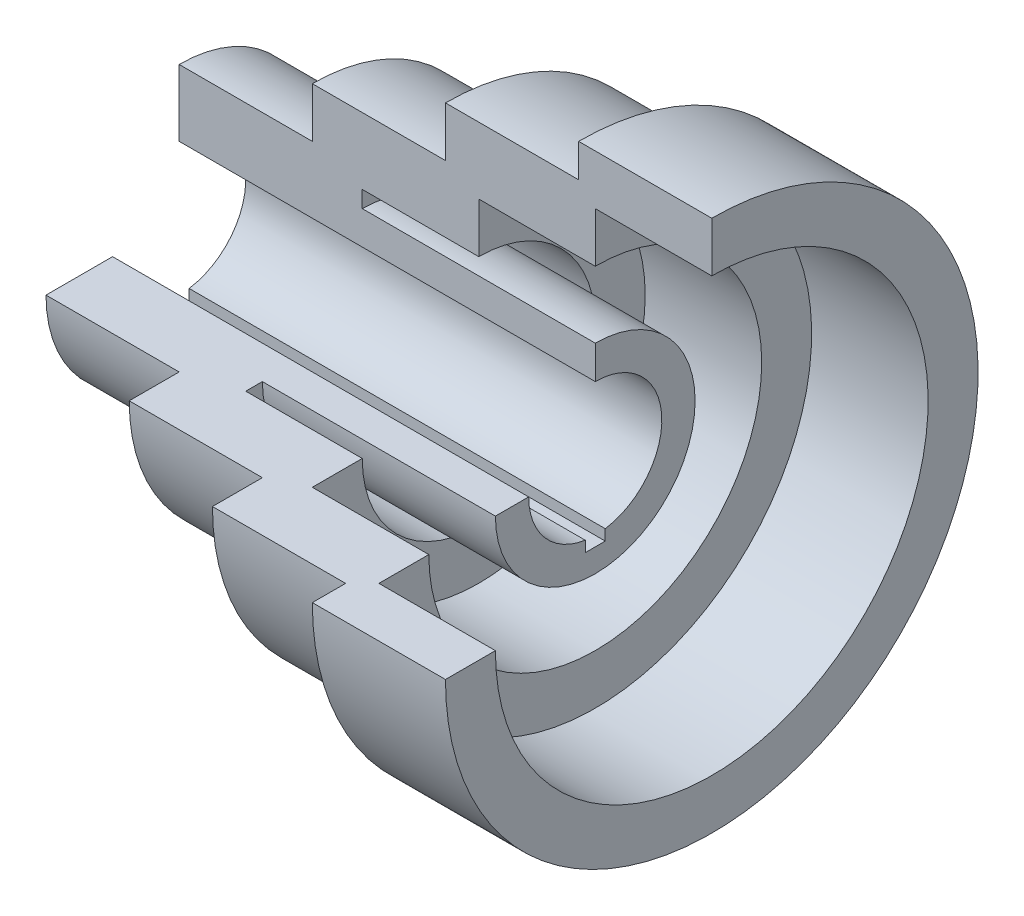
ISO-10303-21;
HEADER;
FILE_DESCRIPTION(('STEP AP214'),'2;1');
FILE_NAME('part.step','',(''),(''),'','','');
FILE_SCHEMA(('AUTOMOTIVE_DESIGN { 1 0 10303 214 1 1 1 1 }'));
ENDSEC;
DATA;
#1=APPLICATION_CONTEXT('core data for automotive mechanical design processes');
#2=APPLICATION_PROTOCOL_DEFINITION('international standard','automotive_design',2000,#1);
#3=PRODUCT_CONTEXT('',#1,'mechanical');
#4=PRODUCT('Part','Part','',(#3));
#5=PRODUCT_RELATED_PRODUCT_CATEGORY('part','',(#4));
#6=PRODUCT_DEFINITION_FORMATION('','',#4);
#7=PRODUCT_DEFINITION_CONTEXT('part definition',#1,'design');
#8=PRODUCT_DEFINITION('design','',#6,#7);
#9=PRODUCT_DEFINITION_SHAPE('','',#8);
#10=(LENGTH_UNIT() NAMED_UNIT(*) SI_UNIT(.MILLI.,.METRE.));
#11=(NAMED_UNIT(*) PLANE_ANGLE_UNIT() SI_UNIT($,.RADIAN.));
#12=(NAMED_UNIT(*) SI_UNIT($,.STERADIAN.) SOLID_ANGLE_UNIT());
#13=UNCERTAINTY_MEASURE_WITH_UNIT(LENGTH_MEASURE(1.E-05),#10,'distance_accuracy_value','');
#14=(GEOMETRIC_REPRESENTATION_CONTEXT(3) GLOBAL_UNCERTAINTY_ASSIGNED_CONTEXT((#13)) GLOBAL_UNIT_ASSIGNED_CONTEXT((#10,
#11,#12)) REPRESENTATION_CONTEXT('',''));
#15=CARTESIAN_POINT('',(0.,0.,0.));
#16=DIRECTION('',(0.,0.,1.));
#17=DIRECTION('',(1.,0.,0.));
#18=AXIS2_PLACEMENT_3D('',#15,#16,#17);
#19=CARTESIAN_POINT('',(125.,0.,0.));
#20=DIRECTION('',(1.,0.,0.));
#21=DIRECTION('',(0.,1.,0.));
#22=AXIS2_PLACEMENT_3D('',#19,#20,#21);
#23=CYLINDRICAL_SURFACE('',#22,20.);
#24=DIRECTION('',(-1.,0.,0.));
#25=VECTOR('',#24,1.);
#26=CARTESIAN_POINT('',(160.,-19.7737199332852,-3.));
#27=LINE('',#26,#25);
#28=CARTESIAN_POINT('',(125.,-19.7737199332852,-3.));
#29=VERTEX_POINT('',#28);
#30=CARTESIAN_POINT('',(0.,-19.7737199332852,-3.));
#31=VERTEX_POINT('',#30);
#32=EDGE_CURVE('E195',#29,#31,#27,.T.);
#33=ORIENTED_EDGE('',*,*,#32,.F.);
#34=CARTESIAN_POINT('',(125.,0.,0.));
#35=DIRECTION('',(1.,0.,0.));
#36=DIRECTION('',(0.,1.,0.));
#37=AXIS2_PLACEMENT_3D('',#34,#35,#36);
#38=CIRCLE('',#37,20.);
#39=CARTESIAN_POINT('',(125.,20.,0.));
#40=VERTEX_POINT('',#39);
#41=EDGE_CURVE('E219',#29,#40,#38,.T.);
#42=ORIENTED_EDGE('',*,*,#41,.T.);
#43=DIRECTION('',(1.,0.,0.));
#44=VECTOR('',#43,1.);
#45=CARTESIAN_POINT('',(0.,20.,0.));
#46=LINE('',#45,#44);
#47=CARTESIAN_POINT('',(0.,20.,0.));
#48=VERTEX_POINT('',#47);
#49=EDGE_CURVE('E212',#48,#40,#46,.T.);
#50=ORIENTED_EDGE('',*,*,#49,.F.);
#51=CARTESIAN_POINT('',(0.,0.,0.));
#52=DIRECTION('',(1.,0.,0.));
#53=DIRECTION('',(0.,1.,0.));
#54=AXIS2_PLACEMENT_3D('',#51,#52,#53);
#55=CIRCLE('',#54,20.);
#56=EDGE_CURVE('E44',#31,#48,#55,.T.);
#57=ORIENTED_EDGE('',*,*,#56,.F.);
#58=EDGE_LOOP('',(#33,#42,#50,#57));
#59=FACE_BOUND('',#58,.T.);
#60=ADVANCED_FACE('F41',(#59),#23,.F.);
#61=CARTESIAN_POINT('',(125.,0.,0.));
#62=DIRECTION('',(1.,0.,0.));
#63=DIRECTION('',(0.,1.,0.));
#64=AXIS2_PLACEMENT_3D('',#61,#62,#63);
#65=PLANE('',#64);
#66=CARTESIAN_POINT('',(125.,0.,0.));
#67=DIRECTION('',(1.,0.,0.));
#68=DIRECTION('',(0.,1.,0.));
#69=AXIS2_PLACEMENT_3D('',#66,#67,#68);
#70=CIRCLE('',#69,65.);
#71=CARTESIAN_POINT('',(125.,6.79104137598434E-13,65.));
#72=VERTEX_POINT('',#71);
#73=CARTESIAN_POINT('',(125.,65.,0.));
#74=VERTEX_POINT('',#73);
#75=EDGE_CURVE('E234',#72,#74,#70,.T.);
#76=ORIENTED_EDGE('',*,*,#75,.T.);
#77=DIRECTION('',(0.,1.,0.));
#78=VECTOR('',#77,1.);
#79=CARTESIAN_POINT('',(125.,0.,0.));
#80=LINE('',#79,#78);
#81=CARTESIAN_POINT('',(125.,50.,0.));
#82=VERTEX_POINT('',#81);
#83=EDGE_CURVE('E209',#82,#74,#80,.T.);
#84=ORIENTED_EDGE('',*,*,#83,.F.);
#85=CARTESIAN_POINT('',(125.,0.,0.));
#86=DIRECTION('',(1.,0.,0.));
#87=DIRECTION('',(0.,1.,0.));
#88=AXIS2_PLACEMENT_3D('',#85,#86,#87);
#89=CIRCLE('',#88,50.);
#90=CARTESIAN_POINT('',(125.,5.21987477350493E-13,50.));
#91=VERTEX_POINT('',#90);
#92=EDGE_CURVE('E70',#91,#82,#89,.T.);
#93=ORIENTED_EDGE('',*,*,#92,.F.);
#94=DIRECTION('',(0.,0.,1.));
#95=VECTOR('',#94,1.);
#96=CARTESIAN_POINT('',(125.,0.,0.));
#97=LINE('',#96,#95);
#98=EDGE_CURVE('E294',#91,#72,#97,.T.);
#99=ORIENTED_EDGE('',*,*,#98,.T.);
#100=EDGE_LOOP('',(#76,#84,#93,#99));
#101=FACE_BOUND('',#100,.T.);
#102=ADVANCED_FACE('F373',(#101),#65,.T.);
#103=CARTESIAN_POINT('',(125.,0.,0.));
#104=DIRECTION('',(1.,0.,0.));
#105=DIRECTION('',(0.,1.,0.));
#106=AXIS2_PLACEMENT_3D('',#103,#104,#105);
#107=CYLINDRICAL_SURFACE('',#106,65.);
#108=CARTESIAN_POINT('',(160.,0.,0.));
#109=DIRECTION('',(1.,0.,0.));
#110=DIRECTION('',(0.,1.,0.));
#111=AXIS2_PLACEMENT_3D('',#108,#109,#110);
#112=CIRCLE('',#111,65.);
#113=CARTESIAN_POINT('',(160.,6.7861841502516E-13,65.));
#114=VERTEX_POINT('',#113);
#115=CARTESIAN_POINT('',(160.,65.,0.));
#116=VERTEX_POINT('',#115);
#117=EDGE_CURVE('E240',#114,#116,#112,.T.);
#118=ORIENTED_EDGE('',*,*,#117,.T.);
#119=DIRECTION('',(1.,0.,0.));
#120=VECTOR('',#119,1.);
#121=CARTESIAN_POINT('',(0.,64.9999999999999,0.));
#122=LINE('',#121,#120);
#123=EDGE_CURVE('E403',#74,#116,#122,.T.);
#124=ORIENTED_EDGE('',*,*,#123,.F.);
#125=ORIENTED_EDGE('',*,*,#75,.F.);
#126=DIRECTION('',(1.,0.,0.));
#127=VECTOR('',#126,1.);
#128=CARTESIAN_POINT('',(0.,6.8083886107441E-13,64.9999999999999));
#129=LINE('',#128,#127);
#130=EDGE_CURVE('E299',#72,#114,#129,.T.);
#131=ORIENTED_EDGE('',*,*,#130,.T.);
#132=EDGE_LOOP('',(#118,#124,#125,#131));
#133=FACE_BOUND('',#132,.T.);
#134=ADVANCED_FACE('F43',(#133),#107,.F.);
#135=CARTESIAN_POINT('',(160.,0.,0.));
#136=DIRECTION('',(-1.,0.,0.));
#137=DIRECTION('',(0.,-1.,0.));
#138=AXIS2_PLACEMENT_3D('',#135,#136,#137);
#139=PLANE('',#138);
#140=CARTESIAN_POINT('',(160.,0.,0.));
#141=DIRECTION('',(1.,0.,0.));
#142=DIRECTION('',(0.,1.,0.));
#143=AXIS2_PLACEMENT_3D('',#140,#141,#142);
#144=CIRCLE('',#143,80.);
#145=CARTESIAN_POINT('',(160.,8.35735075273101E-13,80.));
#146=VERTEX_POINT('',#145);
#147=CARTESIAN_POINT('',(160.,80.,0.));
#148=VERTEX_POINT('',#147);
#149=EDGE_CURVE('E239',#146,#148,#144,.T.);
#150=ORIENTED_EDGE('',*,*,#149,.T.);
#151=DIRECTION('',(0.,-1.,0.));
#152=VECTOR('',#151,1.);
#153=CARTESIAN_POINT('',(160.,0.,0.));
#154=LINE('',#153,#152);
#155=EDGE_CURVE('E406',#148,#116,#154,.T.);
#156=ORIENTED_EDGE('',*,*,#155,.T.);
#157=ORIENTED_EDGE('',*,*,#117,.F.);
#158=DIRECTION('',(0.,0.,-1.));
#159=VECTOR('',#158,1.);
#160=CARTESIAN_POINT('',(160.,0.,0.));
#161=LINE('',#160,#159);
#162=EDGE_CURVE('E298',#146,#114,#161,.T.);
#163=ORIENTED_EDGE('',*,*,#162,.F.);
#164=EDGE_LOOP('',(#150,#156,#157,#163));
#165=FACE_BOUND('',#164,.T.);
#166=ADVANCED_FACE('F455',(#165),#139,.F.);
#167=CARTESIAN_POINT('',(125.,0.,0.));
#168=DIRECTION('',(1.,0.,0.));
#169=DIRECTION('',(0.,1.,0.));
#170=AXIS2_PLACEMENT_3D('',#167,#168,#169);
#171=CYLINDRICAL_SURFACE('',#170,80.);
#172=CARTESIAN_POINT('',(120.,0.,0.));
#173=DIRECTION('',(1.,0.,0.));
#174=DIRECTION('',(0.,1.,0.));
#175=AXIS2_PLACEMENT_3D('',#172,#173,#174);
#176=CIRCLE('',#175,80.);
#177=CARTESIAN_POINT('',(120.,8.36290186785414E-13,80.));
#178=VERTEX_POINT('',#177);
#179=CARTESIAN_POINT('',(120.,80.,0.));
#180=VERTEX_POINT('',#179);
#181=EDGE_CURVE('E244',#178,#180,#176,.T.);
#182=ORIENTED_EDGE('',*,*,#181,.T.);
#183=DIRECTION('',(1.,0.,0.));
#184=VECTOR('',#183,1.);
#185=CARTESIAN_POINT('',(0.,79.9999999999999,0.));
#186=LINE('',#185,#184);
#187=EDGE_CURVE('E412',#180,#148,#186,.T.);
#188=ORIENTED_EDGE('',*,*,#187,.T.);
#189=ORIENTED_EDGE('',*,*,#149,.F.);
#190=DIRECTION('',(1.,0.,0.));
#191=VECTOR('',#190,1.);
#192=CARTESIAN_POINT('',(0.,8.37955521322351E-13,79.9999999999999));
#193=LINE('',#192,#191);
#194=EDGE_CURVE('E305',#178,#146,#193,.T.);
#195=ORIENTED_EDGE('',*,*,#194,.F.);
#196=EDGE_LOOP('',(#182,#188,#189,#195));
#197=FACE_BOUND('',#196,.T.);
#198=ADVANCED_FACE('F450',(#197),#171,.T.);
#199=CARTESIAN_POINT('',(120.,0.,0.));
#200=DIRECTION('',(1.,0.,0.));
#201=DIRECTION('',(0.,1.,0.));
#202=AXIS2_PLACEMENT_3D('',#199,#200,#201);
#203=PLANE('',#202);
#204=CARTESIAN_POINT('',(120.,0.,0.));
#205=DIRECTION('',(1.,0.,0.));
#206=DIRECTION('',(0.,1.,0.));
#207=AXIS2_PLACEMENT_3D('',#204,#205,#206);
#208=CIRCLE('',#207,70.);
#209=CARTESIAN_POINT('',(120.,7.3154574662012E-13,70.));
#210=VERTEX_POINT('',#209);
#211=CARTESIAN_POINT('',(120.,70.,0.));
#212=VERTEX_POINT('',#211);
#213=EDGE_CURVE('E245',#210,#212,#208,.T.);
#214=ORIENTED_EDGE('',*,*,#213,.T.);
#215=DIRECTION('',(0.,1.,0.));
#216=VECTOR('',#215,1.);
#217=CARTESIAN_POINT('',(120.,0.,0.));
#218=LINE('',#217,#216);
#219=EDGE_CURVE('E417',#212,#180,#218,.T.);
#220=ORIENTED_EDGE('',*,*,#219,.T.);
#221=ORIENTED_EDGE('',*,*,#181,.F.);
#222=DIRECTION('',(0.,0.,1.));
#223=VECTOR('',#222,1.);
#224=CARTESIAN_POINT('',(120.,0.,0.));
#225=LINE('',#224,#223);
#226=EDGE_CURVE('E304',#210,#178,#225,.T.);
#227=ORIENTED_EDGE('',*,*,#226,.F.);
#228=EDGE_LOOP('',(#214,#220,#221,#227));
#229=FACE_BOUND('',#228,.T.);
#230=ADVANCED_FACE('F444',(#229),#203,.F.);
#231=CARTESIAN_POINT('',(125.,0.,0.));
#232=DIRECTION('',(1.,0.,0.));
#233=DIRECTION('',(0.,1.,0.));
#234=AXIS2_PLACEMENT_3D('',#231,#232,#233);
#235=CYLINDRICAL_SURFACE('',#234,70.);
#236=CARTESIAN_POINT('',(80.,0.,0.));
#237=DIRECTION('',(1.,0.,0.));
#238=DIRECTION('',(0.,1.,0.));
#239=AXIS2_PLACEMENT_3D('',#236,#237,#238);
#240=CIRCLE('',#239,70.);
#241=CARTESIAN_POINT('',(80.,7.32100858132433E-13,70.));
#242=VERTEX_POINT('',#241);
#243=CARTESIAN_POINT('',(80.,70.,0.));
#244=VERTEX_POINT('',#243);
#245=EDGE_CURVE('E242',#242,#244,#240,.T.);
#246=ORIENTED_EDGE('',*,*,#245,.T.);
#247=DIRECTION('',(1.,0.,0.));
#248=VECTOR('',#247,1.);
#249=CARTESIAN_POINT('',(0.,69.9999999999999,0.));
#250=LINE('',#249,#248);
#251=EDGE_CURVE('E419',#244,#212,#250,.T.);
#252=ORIENTED_EDGE('',*,*,#251,.T.);
#253=ORIENTED_EDGE('',*,*,#213,.F.);
#254=DIRECTION('',(1.,0.,0.));
#255=VECTOR('',#254,1.);
#256=CARTESIAN_POINT('',(0.,7.33211081157057E-13,69.9999999999999));
#257=LINE('',#256,#255);
#258=EDGE_CURVE('E306',#242,#210,#257,.T.);
#259=ORIENTED_EDGE('',*,*,#258,.F.);
#260=EDGE_LOOP('',(#246,#252,#253,#259));
#261=FACE_BOUND('',#260,.T.);
#262=ADVANCED_FACE('F438',(#261),#235,.T.);
#263=CARTESIAN_POINT('',(80.,0.,0.));
#264=DIRECTION('',(1.,0.,0.));
#265=DIRECTION('',(0.,1.,0.));
#266=AXIS2_PLACEMENT_3D('',#263,#264,#265);
#267=PLANE('',#266);
#268=CARTESIAN_POINT('',(80.,0.,0.));
#269=DIRECTION('',(1.,0.,0.));
#270=DIRECTION('',(0.,1.,0.));
#271=AXIS2_PLACEMENT_3D('',#268,#269,#270);
#272=CIRCLE('',#271,55.);
#273=CARTESIAN_POINT('',(80.,5.74984197884491E-13,55.));
#274=VERTEX_POINT('',#273);
#275=CARTESIAN_POINT('',(80.,55.,0.));
#276=VERTEX_POINT('',#275);
#277=EDGE_CURVE('E250',#274,#276,#272,.T.);
#278=ORIENTED_EDGE('',*,*,#277,.T.);
#279=DIRECTION('',(0.,1.,0.));
#280=VECTOR('',#279,1.);
#281=CARTESIAN_POINT('',(80.,0.,0.));
#282=LINE('',#281,#280);
#283=EDGE_CURVE('E421',#276,#244,#282,.T.);
#284=ORIENTED_EDGE('',*,*,#283,.T.);
#285=ORIENTED_EDGE('',*,*,#245,.F.);
#286=DIRECTION('',(0.,0.,1.));
#287=VECTOR('',#286,1.);
#288=CARTESIAN_POINT('',(80.,0.,0.));
#289=LINE('',#288,#287);
#290=EDGE_CURVE('E313',#274,#242,#289,.T.);
#291=ORIENTED_EDGE('',*,*,#290,.F.);
#292=EDGE_LOOP('',(#278,#284,#285,#291));
#293=FACE_BOUND('',#292,.T.);
#294=ADVANCED_FACE('F434',(#293),#267,.F.);
#295=CARTESIAN_POINT('',(125.,0.,0.));
#296=DIRECTION('',(1.,0.,0.));
#297=DIRECTION('',(0.,1.,0.));
#298=AXIS2_PLACEMENT_3D('',#295,#296,#297);
#299=CYLINDRICAL_SURFACE('',#298,55.);
#300=CARTESIAN_POINT('',(40.,0.,0.));
#301=DIRECTION('',(1.,0.,0.));
#302=DIRECTION('',(0.,1.,0.));
#303=AXIS2_PLACEMENT_3D('',#300,#301,#302);
#304=CIRCLE('',#303,55.);
#305=CARTESIAN_POINT('',(40.,5.75539309396804E-13,55.));
#306=VERTEX_POINT('',#305);
#307=CARTESIAN_POINT('',(40.,55.,0.));
#308=VERTEX_POINT('',#307);
#309=EDGE_CURVE('E247',#306,#308,#304,.T.);
#310=ORIENTED_EDGE('',*,*,#309,.T.);
#311=DIRECTION('',(1.,0.,0.));
#312=VECTOR('',#311,1.);
#313=CARTESIAN_POINT('',(0.,55.,0.));
#314=LINE('',#313,#312);
#315=EDGE_CURVE('E426',#308,#276,#314,.T.);
#316=ORIENTED_EDGE('',*,*,#315,.T.);
#317=ORIENTED_EDGE('',*,*,#277,.F.);
#318=DIRECTION('',(1.,0.,0.));
#319=VECTOR('',#318,1.);
#320=CARTESIAN_POINT('',(0.,5.76094420909117E-13,55.));
#321=LINE('',#320,#319);
#322=EDGE_CURVE('E314',#306,#274,#321,.T.);
#323=ORIENTED_EDGE('',*,*,#322,.F.);
#324=EDGE_LOOP('',(#310,#316,#317,#323));
#325=FACE_BOUND('',#324,.T.);
#326=ADVANCED_FACE('F431',(#325),#299,.T.);
#327=CARTESIAN_POINT('',(40.,0.,0.));
#328=DIRECTION('',(1.,0.,0.));
#329=DIRECTION('',(0.,1.,0.));
#330=AXIS2_PLACEMENT_3D('',#327,#328,#329);
#331=PLANE('',#330);
#332=CARTESIAN_POINT('',(40.,0.,0.));
#333=DIRECTION('',(1.,0.,0.));
#334=DIRECTION('',(0.,1.,0.));
#335=AXIS2_PLACEMENT_3D('',#332,#333,#334);
#336=CIRCLE('',#335,40.);
#337=CARTESIAN_POINT('',(40.,4.18422649148863E-13,40.));
#338=VERTEX_POINT('',#337);
#339=CARTESIAN_POINT('',(40.,40.,0.));
#340=VERTEX_POINT('',#339);
#341=EDGE_CURVE('E249',#338,#340,#336,.T.);
#342=ORIENTED_EDGE('',*,*,#341,.T.);
#343=DIRECTION('',(0.,1.,0.));
#344=VECTOR('',#343,1.);
#345=CARTESIAN_POINT('',(40.,0.,0.));
#346=LINE('',#345,#344);
#347=EDGE_CURVE('E269',#340,#308,#346,.T.);
#348=ORIENTED_EDGE('',*,*,#347,.T.);
#349=ORIENTED_EDGE('',*,*,#309,.F.);
#350=DIRECTION('',(0.,0.,1.));
#351=VECTOR('',#350,1.);
#352=CARTESIAN_POINT('',(40.,0.,0.));
#353=LINE('',#352,#351);
#354=EDGE_CURVE('E320',#338,#306,#353,.T.);
#355=ORIENTED_EDGE('',*,*,#354,.F.);
#356=EDGE_LOOP('',(#342,#348,#349,#355));
#357=FACE_BOUND('',#356,.T.);
#358=ADVANCED_FACE('F428',(#357),#331,.F.);
#359=CARTESIAN_POINT('',(125.,0.,0.));
#360=DIRECTION('',(1.,0.,0.));
#361=DIRECTION('',(0.,1.,0.));
#362=AXIS2_PLACEMENT_3D('',#359,#360,#361);
#363=CYLINDRICAL_SURFACE('',#362,40.);
#364=CARTESIAN_POINT('',(0.,0.,0.));
#365=DIRECTION('',(1.,0.,0.));
#366=DIRECTION('',(0.,1.,0.));
#367=AXIS2_PLACEMENT_3D('',#364,#365,#366);
#368=CIRCLE('',#367,40.);
#369=CARTESIAN_POINT('',(0.,4.18977760661176E-13,40.));
#370=VERTEX_POINT('',#369);
#371=CARTESIAN_POINT('',(0.,40.,0.));
#372=VERTEX_POINT('',#371);
#373=EDGE_CURVE('E217',#370,#372,#368,.T.);
#374=ORIENTED_EDGE('',*,*,#373,.T.);
#375=DIRECTION('',(1.,0.,0.));
#376=VECTOR('',#375,1.);
#377=CARTESIAN_POINT('',(0.,40.,0.));
#378=LINE('',#377,#376);
#379=EDGE_CURVE('E257',#372,#340,#378,.T.);
#380=ORIENTED_EDGE('',*,*,#379,.T.);
#381=ORIENTED_EDGE('',*,*,#341,.F.);
#382=DIRECTION('',(1.,0.,0.));
#383=VECTOR('',#382,1.);
#384=CARTESIAN_POINT('',(0.,4.18977760661176E-13,40.));
#385=LINE('',#384,#383);
#386=EDGE_CURVE('E265',#370,#338,#385,.T.);
#387=ORIENTED_EDGE('',*,*,#386,.F.);
#388=EDGE_LOOP('',(#374,#380,#381,#387));
#389=FACE_BOUND('',#388,.T.);
#390=ADVANCED_FACE('F259',(#389),#363,.T.);
#391=CARTESIAN_POINT('',(0.,0.,0.));
#392=DIRECTION('',(1.,0.,0.));
#393=DIRECTION('',(0.,1.,0.));
#394=AXIS2_PLACEMENT_3D('',#391,#392,#393);
#395=PLANE('',#394);
#396=DIRECTION('',(0.,0.,-1.));
#397=VECTOR('',#396,1.);
#398=CARTESIAN_POINT('',(0.,-23.,0.));
#399=LINE('',#398,#397);
#400=CARTESIAN_POINT('',(0.,-23.,3.));
#401=VERTEX_POINT('',#400);
#402=CARTESIAN_POINT('',(0.,-23.,-3.));
#403=VERTEX_POINT('',#402);
#404=EDGE_CURVE('E207',#401,#403,#399,.T.);
#405=ORIENTED_EDGE('',*,*,#404,.T.);
#406=DIRECTION('',(0.,1.,0.));
#407=VECTOR('',#406,1.);
#408=CARTESIAN_POINT('',(0.,0.,-3.));
#409=LINE('',#408,#407);
#410=EDGE_CURVE('E198',#403,#31,#409,.T.);
#411=ORIENTED_EDGE('',*,*,#410,.T.);
#412=ORIENTED_EDGE('',*,*,#56,.T.);
#413=DIRECTION('',(0.,1.,0.));
#414=VECTOR('',#413,1.);
#415=CARTESIAN_POINT('',(0.,0.,0.));
#416=LINE('',#415,#414);
#417=EDGE_CURVE('E268',#48,#372,#416,.T.);
#418=ORIENTED_EDGE('',*,*,#417,.T.);
#419=ORIENTED_EDGE('',*,*,#373,.F.);
#420=DIRECTION('',(0.,0.,1.));
#421=VECTOR('',#420,1.);
#422=CARTESIAN_POINT('',(0.,0.,0.));
#423=LINE('',#422,#421);
#424=CARTESIAN_POINT('',(0.,2.09488880330588E-13,20.));
#425=VERTEX_POINT('',#424);
#426=EDGE_CURVE('E321',#425,#370,#423,.T.);
#427=ORIENTED_EDGE('',*,*,#426,.F.);
#428=CARTESIAN_POINT('',(-6.E-06,-19.7737199332852,3.));
#429=VERTEX_POINT('',#428);
#430=EDGE_CURVE('E214',#425,#429,#55,.T.);
#431=ORIENTED_EDGE('',*,*,#430,.T.);
#432=DIRECTION('',(0.,-1.,0.));
#433=VECTOR('',#432,1.);
#434=CARTESIAN_POINT('',(0.,0.,3.));
#435=LINE('',#434,#433);
#436=EDGE_CURVE('E390',#429,#401,#435,.T.);
#437=ORIENTED_EDGE('',*,*,#436,.T.);
#438=EDGE_LOOP('',(#405,#411,#412,#418,#419,#427,#431,#437));
#439=FACE_BOUND('',#438,.T.);
#440=ADVANCED_FACE('F202',(#439),#395,.F.);
#441=DIRECTION('',(-1.,0.,0.));
#442=VECTOR('',#441,1.);
#443=CARTESIAN_POINT('',(160.,-19.7737199332852,3.));
#444=LINE('',#443,#442);
#445=CARTESIAN_POINT('',(125.,-19.7737199332852,3.));
#446=VERTEX_POINT('',#445);
#447=EDGE_CURVE('E56',#446,#429,#444,.T.);
#448=ORIENTED_EDGE('',*,*,#447,.T.);
#449=ORIENTED_EDGE('',*,*,#430,.F.);
#450=DIRECTION('',(1.,0.,0.));
#451=VECTOR('',#450,1.);
#452=CARTESIAN_POINT('',(0.,2.09488880330588E-13,20.));
#453=LINE('',#452,#451);
#454=CARTESIAN_POINT('',(125.,2.07754156854611E-13,20.));
#455=VERTEX_POINT('',#454);
#456=EDGE_CURVE('E323',#425,#455,#453,.T.);
#457=ORIENTED_EDGE('',*,*,#456,.T.);
#458=EDGE_CURVE('E216',#455,#446,#38,.T.);
#459=ORIENTED_EDGE('',*,*,#458,.T.);
#460=EDGE_LOOP('',(#448,#449,#457,#459));
#461=FACE_BOUND('',#460,.T.);
#462=ADVANCED_FACE('F367',(#461),#23,.F.);
#463=CARTESIAN_POINT('',(125.,0.,0.));
#464=DIRECTION('',(1.,0.,0.));
#465=DIRECTION('',(0.,1.,0.));
#466=AXIS2_PLACEMENT_3D('',#463,#464,#465);
#467=PLANE('',#466);
#468=DIRECTION('',(0.,1.,0.));
#469=VECTOR('',#468,1.);
#470=CARTESIAN_POINT('',(125.,0.,-3.));
#471=LINE('',#470,#469);
#472=CARTESIAN_POINT('',(125.,-23.,-3.));
#473=VERTEX_POINT('',#472);
#474=EDGE_CURVE('E11',#473,#29,#471,.T.);
#475=ORIENTED_EDGE('',*,*,#474,.F.);
#476=DIRECTION('',(0.,0.,-1.));
#477=VECTOR('',#476,1.);
#478=CARTESIAN_POINT('',(125.,-23.,0.));
#479=LINE('',#478,#477);
#480=CARTESIAN_POINT('',(125.,-23.,3.));
#481=VERTEX_POINT('',#480);
#482=EDGE_CURVE('E51',#481,#473,#479,.T.);
#483=ORIENTED_EDGE('',*,*,#482,.F.);
#484=DIRECTION('',(0.,-1.,0.));
#485=VECTOR('',#484,1.);
#486=CARTESIAN_POINT('',(125.,0.,3.));
#487=LINE('',#486,#485);
#488=EDGE_CURVE('E233',#446,#481,#487,.T.);
#489=ORIENTED_EDGE('',*,*,#488,.F.);
#490=ORIENTED_EDGE('',*,*,#458,.F.);
#491=DIRECTION('',(0.,0.,1.));
#492=VECTOR('',#491,1.);
#493=CARTESIAN_POINT('',(125.,0.,0.));
#494=LINE('',#493,#492);
#495=CARTESIAN_POINT('',(125.,3.12498597019905E-13,30.));
#496=VERTEX_POINT('',#495);
#497=EDGE_CURVE('E324',#455,#496,#494,.T.);
#498=ORIENTED_EDGE('',*,*,#497,.T.);
#499=CARTESIAN_POINT('',(125.,0.,0.));
#500=DIRECTION('',(1.,0.,0.));
#501=DIRECTION('',(0.,1.,0.));
#502=AXIS2_PLACEMENT_3D('',#499,#500,#501);
#503=CIRCLE('',#502,30.);
#504=CARTESIAN_POINT('',(125.,30.,0.));
#505=VERTEX_POINT('',#504);
#506=EDGE_CURVE('E221',#496,#505,#503,.T.);
#507=ORIENTED_EDGE('',*,*,#506,.T.);
#508=DIRECTION('',(0.,1.,0.));
#509=VECTOR('',#508,1.);
#510=CARTESIAN_POINT('',(125.,0.,0.));
#511=LINE('',#510,#509);
#512=EDGE_CURVE('E272',#40,#505,#511,.T.);
#513=ORIENTED_EDGE('',*,*,#512,.F.);
#514=ORIENTED_EDGE('',*,*,#41,.F.);
#515=EDGE_LOOP('',(#475,#483,#489,#490,#498,#507,#513,#514));
#516=FACE_BOUND('',#515,.T.);
#517=ADVANCED_FACE('F353',(#516),#467,.T.);
#518=CARTESIAN_POINT('',(125.,0.,0.));
#519=DIRECTION('',(1.,0.,0.));
#520=DIRECTION('',(0.,1.,0.));
#521=AXIS2_PLACEMENT_3D('',#518,#519,#520);
#522=CYLINDRICAL_SURFACE('',#521,30.);
#523=CARTESIAN_POINT('',(55.,0.,0.));
#524=DIRECTION('',(1.,0.,0.));
#525=DIRECTION('',(0.,1.,0.));
#526=AXIS2_PLACEMENT_3D('',#523,#524,#525);
#527=CIRCLE('',#526,30.);
#528=CARTESIAN_POINT('',(55.,3.13470042166452E-13,30.));
#529=VERTEX_POINT('',#528);
#530=CARTESIAN_POINT('',(55.,30.,0.));
#531=VERTEX_POINT('',#530);
#532=EDGE_CURVE('E349',#529,#531,#527,.T.);
#533=ORIENTED_EDGE('',*,*,#532,.T.);
#534=DIRECTION('',(-1.,0.,0.));
#535=VECTOR('',#534,1.);
#536=CARTESIAN_POINT('',(0.,30.,0.));
#537=LINE('',#536,#535);
#538=EDGE_CURVE('E276',#505,#531,#537,.T.);
#539=ORIENTED_EDGE('',*,*,#538,.F.);
#540=ORIENTED_EDGE('',*,*,#506,.F.);
#541=DIRECTION('',(-1.,0.,0.));
#542=VECTOR('',#541,1.);
#543=CARTESIAN_POINT('',(0.,3.14233320495881E-13,30.));
#544=LINE('',#543,#542);
#545=EDGE_CURVE('E327',#496,#529,#544,.T.);
#546=ORIENTED_EDGE('',*,*,#545,.T.);
#547=EDGE_LOOP('',(#533,#539,#540,#546));
#548=FACE_BOUND('',#547,.T.);
#549=ADVANCED_FACE('F358',(#548),#522,.T.);
#550=CARTESIAN_POINT('',(55.,0.,0.));
#551=DIRECTION('',(1.,0.,0.));
#552=DIRECTION('',(0.,1.,0.));
#553=AXIS2_PLACEMENT_3D('',#550,#551,#552);
#554=PLANE('',#553);
#555=CARTESIAN_POINT('',(55.,0.,0.));
#556=DIRECTION('',(1.,0.,0.));
#557=DIRECTION('',(0.,1.,0.));
#558=AXIS2_PLACEMENT_3D('',#555,#556,#557);
#559=CIRCLE('',#558,35.);
#560=CARTESIAN_POINT('',(55.,3.65842262249099E-13,35.));
#561=VERTEX_POINT('',#560);
#562=CARTESIAN_POINT('',(55.,35.,0.));
#563=VERTEX_POINT('',#562);
#564=EDGE_CURVE('E346',#561,#563,#559,.T.);
#565=ORIENTED_EDGE('',*,*,#564,.T.);
#566=DIRECTION('',(0.,1.,0.));
#567=VECTOR('',#566,1.);
#568=CARTESIAN_POINT('',(55.,0.,0.));
#569=LINE('',#568,#567);
#570=EDGE_CURVE('E281',#531,#563,#569,.T.);
#571=ORIENTED_EDGE('',*,*,#570,.F.);
#572=ORIENTED_EDGE('',*,*,#532,.F.);
#573=DIRECTION('',(0.,0.,1.));
#574=VECTOR('',#573,1.);
#575=CARTESIAN_POINT('',(55.,0.,0.));
#576=LINE('',#575,#574);
#577=EDGE_CURVE('E332',#529,#561,#576,.T.);
#578=ORIENTED_EDGE('',*,*,#577,.T.);
#579=EDGE_LOOP('',(#565,#571,#572,#578));
#580=FACE_BOUND('',#579,.T.);
#581=ADVANCED_FACE('F359',(#580),#554,.T.);
#582=CARTESIAN_POINT('',(125.,0.,0.));
#583=DIRECTION('',(1.,0.,0.));
#584=DIRECTION('',(0.,1.,0.));
#585=AXIS2_PLACEMENT_3D('',#582,#583,#584);
#586=CYLINDRICAL_SURFACE('',#585,35.);
#587=CARTESIAN_POINT('',(90.,0.,0.));
#588=DIRECTION('',(1.,0.,0.));
#589=DIRECTION('',(0.,1.,0.));
#590=AXIS2_PLACEMENT_3D('',#587,#588,#589);
#591=CIRCLE('',#590,35.);
#592=CARTESIAN_POINT('',(90.,3.65356539675825E-13,35.));
#593=VERTEX_POINT('',#592);
#594=CARTESIAN_POINT('',(90.,35.,0.));
#595=VERTEX_POINT('',#594);
#596=EDGE_CURVE('E347',#593,#595,#591,.T.);
#597=ORIENTED_EDGE('',*,*,#596,.T.);
#598=DIRECTION('',(1.,0.,0.));
#599=VECTOR('',#598,1.);
#600=CARTESIAN_POINT('',(0.,35.,0.));
#601=LINE('',#600,#599);
#602=EDGE_CURVE('E282',#563,#595,#601,.T.);
#603=ORIENTED_EDGE('',*,*,#602,.F.);
#604=ORIENTED_EDGE('',*,*,#564,.F.);
#605=DIRECTION('',(1.,0.,0.));
#606=VECTOR('',#605,1.);
#607=CARTESIAN_POINT('',(0.,3.66605540578529E-13,35.));
#608=LINE('',#607,#606);
#609=EDGE_CURVE('E331',#561,#593,#608,.T.);
#610=ORIENTED_EDGE('',*,*,#609,.T.);
#611=EDGE_LOOP('',(#597,#603,#604,#610));
#612=FACE_BOUND('',#611,.T.);
#613=ADVANCED_FACE('F368',(#612),#586,.F.);
#614=CARTESIAN_POINT('',(90.,0.,0.));
#615=DIRECTION('',(1.,0.,0.));
#616=DIRECTION('',(0.,1.,0.));
#617=AXIS2_PLACEMENT_3D('',#614,#615,#616);
#618=PLANE('',#617);
#619=CARTESIAN_POINT('',(90.,0.,0.));
#620=DIRECTION('',(1.,0.,0.));
#621=DIRECTION('',(0.,1.,0.));
#622=AXIS2_PLACEMENT_3D('',#619,#620,#621);
#623=CIRCLE('',#622,50.);
#624=CARTESIAN_POINT('',(90.,5.22473199923766E-13,50.));
#625=VERTEX_POINT('',#624);
#626=CARTESIAN_POINT('',(90.,50.,0.));
#627=VERTEX_POINT('',#626);
#628=EDGE_CURVE('E342',#625,#627,#623,.T.);
#629=ORIENTED_EDGE('',*,*,#628,.T.);
#630=DIRECTION('',(0.,1.,0.));
#631=VECTOR('',#630,1.);
#632=CARTESIAN_POINT('',(90.,0.,0.));
#633=LINE('',#632,#631);
#634=EDGE_CURVE('E288',#595,#627,#633,.T.);
#635=ORIENTED_EDGE('',*,*,#634,.F.);
#636=ORIENTED_EDGE('',*,*,#596,.F.);
#637=DIRECTION('',(0.,0.,1.));
#638=VECTOR('',#637,1.);
#639=CARTESIAN_POINT('',(90.,0.,0.));
#640=LINE('',#639,#638);
#641=EDGE_CURVE('E336',#593,#625,#640,.T.);
#642=ORIENTED_EDGE('',*,*,#641,.T.);
#643=EDGE_LOOP('',(#629,#635,#636,#642));
#644=FACE_BOUND('',#643,.T.);
#645=ADVANCED_FACE('F398',(#644),#618,.T.);
#646=CARTESIAN_POINT('',(125.,0.,0.));
#647=DIRECTION('',(1.,0.,0.));
#648=DIRECTION('',(0.,1.,0.));
#649=AXIS2_PLACEMENT_3D('',#646,#647,#648);
#650=CYLINDRICAL_SURFACE('',#649,50.);
#651=DIRECTION('',(1.,0.,0.));
#652=VECTOR('',#651,1.);
#653=CARTESIAN_POINT('',(0.,5.2372220082647E-13,50.));
#654=LINE('',#653,#652);
#655=EDGE_CURVE('E337',#625,#91,#654,.T.);
#656=ORIENTED_EDGE('',*,*,#655,.T.);
#657=ORIENTED_EDGE('',*,*,#92,.T.);
#658=DIRECTION('',(1.,0.,0.));
#659=VECTOR('',#658,1.);
#660=CARTESIAN_POINT('',(0.,50.,0.));
#661=LINE('',#660,#659);
#662=EDGE_CURVE('E292',#627,#82,#661,.T.);
#663=ORIENTED_EDGE('',*,*,#662,.F.);
#664=ORIENTED_EDGE('',*,*,#628,.F.);
#665=EDGE_LOOP('',(#656,#657,#663,#664));
#666=FACE_BOUND('',#665,.T.);
#667=ADVANCED_FACE('F405',(#666),#650,.F.);
#668=CARTESIAN_POINT('',(0.,0.,0.));
#669=DIRECTION('',(0.,-1.,0.));
#670=DIRECTION('',(1.,0.,0.));
#671=AXIS2_PLACEMENT_3D('',#668,#669,#670);
#672=PLANE('',#671);
#673=ORIENTED_EDGE('',*,*,#98,.F.);
#674=ORIENTED_EDGE('',*,*,#655,.F.);
#675=ORIENTED_EDGE('',*,*,#641,.F.);
#676=ORIENTED_EDGE('',*,*,#609,.F.);
#677=ORIENTED_EDGE('',*,*,#577,.F.);
#678=ORIENTED_EDGE('',*,*,#545,.F.);
#679=ORIENTED_EDGE('',*,*,#497,.F.);
#680=ORIENTED_EDGE('',*,*,#456,.F.);
#681=ORIENTED_EDGE('',*,*,#426,.T.);
#682=ORIENTED_EDGE('',*,*,#386,.T.);
#683=ORIENTED_EDGE('',*,*,#354,.T.);
#684=ORIENTED_EDGE('',*,*,#322,.T.);
#685=ORIENTED_EDGE('',*,*,#290,.T.);
#686=ORIENTED_EDGE('',*,*,#258,.T.);
#687=ORIENTED_EDGE('',*,*,#226,.T.);
#688=ORIENTED_EDGE('',*,*,#194,.T.);
#689=ORIENTED_EDGE('',*,*,#162,.T.);
#690=ORIENTED_EDGE('',*,*,#130,.F.);
#691=EDGE_LOOP('',(#673,#674,#675,#676,#677,#678,#679,#680,#681,#682,#683,#684,#685,#686,#687,
#688,#689,#690));
#692=FACE_BOUND('',#691,.T.);
#693=ADVANCED_FACE('F388',(#692),#672,.F.);
#694=CARTESIAN_POINT('',(0.,0.,0.));
#695=DIRECTION('',(0.,0.,1.));
#696=DIRECTION('',(1.,0.,0.));
#697=AXIS2_PLACEMENT_3D('',#694,#695,#696);
#698=PLANE('',#697);
#699=ORIENTED_EDGE('',*,*,#83,.T.);
#700=ORIENTED_EDGE('',*,*,#123,.T.);
#701=ORIENTED_EDGE('',*,*,#155,.F.);
#702=ORIENTED_EDGE('',*,*,#187,.F.);
#703=ORIENTED_EDGE('',*,*,#219,.F.);
#704=ORIENTED_EDGE('',*,*,#251,.F.);
#705=ORIENTED_EDGE('',*,*,#283,.F.);
#706=ORIENTED_EDGE('',*,*,#315,.F.);
#707=ORIENTED_EDGE('',*,*,#347,.F.);
#708=ORIENTED_EDGE('',*,*,#379,.F.);
#709=ORIENTED_EDGE('',*,*,#417,.F.);
#710=ORIENTED_EDGE('',*,*,#49,.T.);
#711=ORIENTED_EDGE('',*,*,#512,.T.);
#712=ORIENTED_EDGE('',*,*,#538,.T.);
#713=ORIENTED_EDGE('',*,*,#570,.T.);
#714=ORIENTED_EDGE('',*,*,#602,.T.);
#715=ORIENTED_EDGE('',*,*,#634,.T.);
#716=ORIENTED_EDGE('',*,*,#662,.T.);
#717=EDGE_LOOP('',(#699,#700,#701,#702,#703,#704,#705,#706,#707,#708,#709,#710,#711,#712,#713,
#714,#715,#716));
#718=FACE_BOUND('',#717,.T.);
#719=ADVANCED_FACE('F270',(#718),#698,.T.);
#720=CARTESIAN_POINT('',(-1.2E-05,0.,-3.));
#721=DIRECTION('',(0.,0.,-1.));
#722=DIRECTION('',(-1.,0.,0.));
#723=AXIS2_PLACEMENT_3D('',#720,#721,#722);
#724=PLANE('',#723);
#725=DIRECTION('',(1.,0.,0.));
#726=VECTOR('',#725,1.);
#727=CARTESIAN_POINT('',(-1.2E-05,-23.,-3.));
#728=LINE('',#727,#726);
#729=EDGE_CURVE('E624',#403,#473,#728,.T.);
#730=ORIENTED_EDGE('',*,*,#729,.T.);
#731=ORIENTED_EDGE('',*,*,#474,.T.);
#732=ORIENTED_EDGE('',*,*,#32,.T.);
#733=ORIENTED_EDGE('',*,*,#410,.F.);
#734=EDGE_LOOP('',(#730,#731,#732,#733));
#735=FACE_BOUND('',#734,.T.);
#736=ADVANCED_FACE('F194',(#735),#724,.F.);
#737=CARTESIAN_POINT('',(-1.2E-05,-23.,0.));
#738=DIRECTION('',(0.,-1.,0.));
#739=DIRECTION('',(0.,0.,-1.));
#740=AXIS2_PLACEMENT_3D('',#737,#738,#739);
#741=PLANE('',#740);
#742=DIRECTION('',(1.,0.,0.));
#743=VECTOR('',#742,1.);
#744=CARTESIAN_POINT('',(-1.2E-05,-23.,3.));
#745=LINE('',#744,#743);
#746=EDGE_CURVE('E384',#401,#481,#745,.T.);
#747=ORIENTED_EDGE('',*,*,#746,.T.);
#748=ORIENTED_EDGE('',*,*,#482,.T.);
#749=ORIENTED_EDGE('',*,*,#729,.F.);
#750=ORIENTED_EDGE('',*,*,#404,.F.);
#751=EDGE_LOOP('',(#747,#748,#749,#750));
#752=FACE_BOUND('',#751,.T.);
#753=ADVANCED_FACE('F594',(#752),#741,.F.);
#754=CARTESIAN_POINT('',(-1.2E-05,0.,3.));
#755=DIRECTION('',(0.,0.,1.));
#756=DIRECTION('',(0.,-1.,0.));
#757=AXIS2_PLACEMENT_3D('',#754,#755,#756);
#758=PLANE('',#757);
#759=ORIENTED_EDGE('',*,*,#447,.F.);
#760=ORIENTED_EDGE('',*,*,#488,.T.);
#761=ORIENTED_EDGE('',*,*,#746,.F.);
#762=ORIENTED_EDGE('',*,*,#436,.F.);
#763=EDGE_LOOP('',(#759,#760,#761,#762));
#764=FACE_BOUND('',#763,.T.);
#765=ADVANCED_FACE('F602',(#764),#758,.F.);
#766=CLOSED_SHELL('',(#60,#102,#134,#166,#198,#230,#262,#294,#326,#358,#390,#440,#462,#517,#549,
#581,#613,#645,#667,#693,#719,#736,#753,#765));
#767=MANIFOLD_SOLID_BREP('B2',#766);
#768=ADVANCED_BREP_SHAPE_REPRESENTATION('',(#18,#767),#14);
#769=SHAPE_DEFINITION_REPRESENTATION(#9,#768);
ENDSEC;
END-ISO-10303-21;
